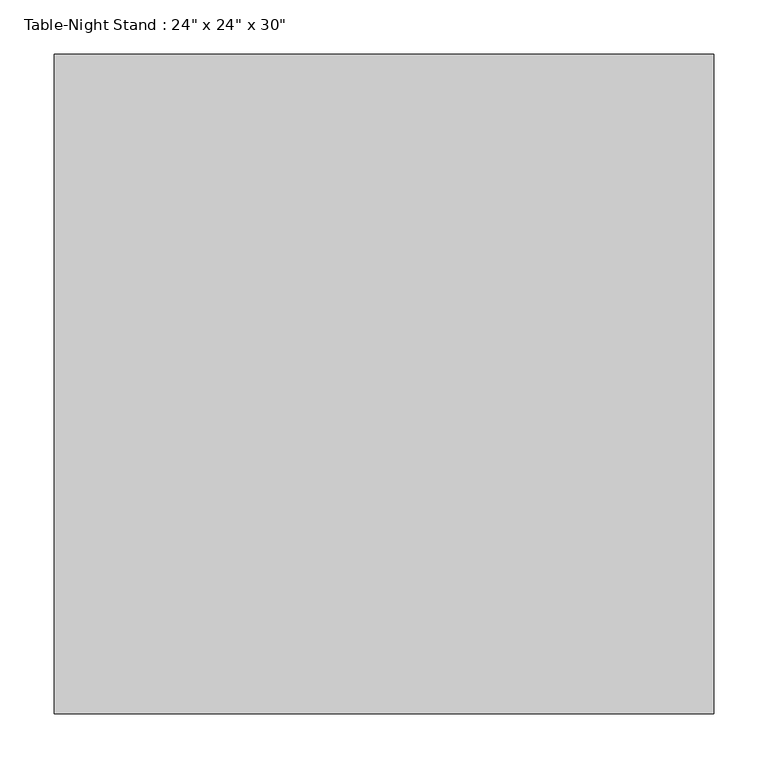
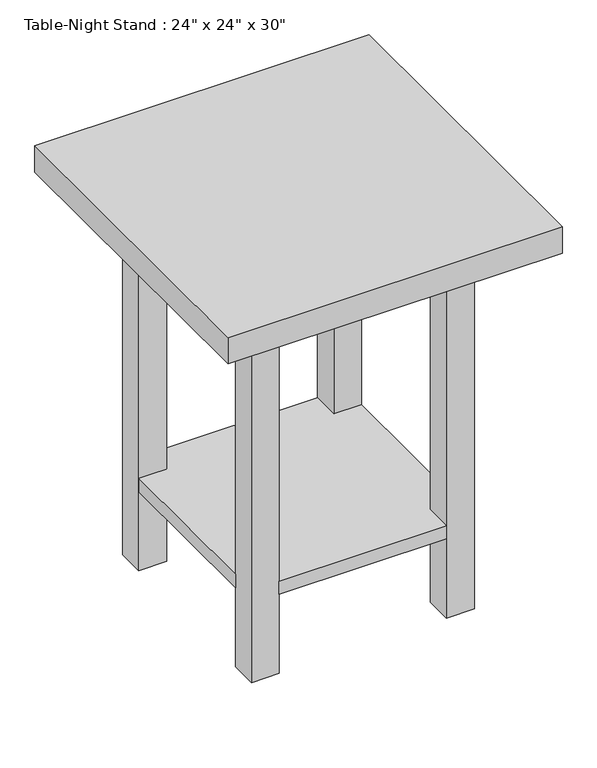
"""IFC4 building model written with IfcOpenShell, lengths in millimetres: furniture geometry."""

from ifc_helpers import new_model, si_unit, frame, origin, origin_with_axes, place, context, project, spatial, polyline, outline, extrude, source, transform, mapped, element, save


def furniture_5bc9ed15(model_context):
    return source(origin(), model_context, "Body", "SweptSolid", [
        extrude(outline(polyline([(156.1336303, 508.0), (460.9336303, 508.0), (460.9336303, 457.2), (511.7336303, 457.2), (511.7336303, 152.4), (460.9336303, 152.4), (460.9336303, 101.6), (156.1336303, 101.6), (156.1336303, 152.4), (105.3336303, 152.4), (105.3336303, 457.2), (156.1336303, 457.2), (156.1336303, 508.0)])), frame((0.0, 0.0, 152.4), z_axis=(0.0, 0.0, 1.0), x_axis=(1.0, 0.0, 0.0)), (0.0, 0.0, 1.0), 25.4),
        extrude(outline(polyline([(156.1336303, 508.0), (156.1336303, 457.2), (105.3336303, 457.2), (105.3336303, 508.0), (156.1336303, 508.0)])), origin_with_axes(), (0.0, 0.0, 1.0), 711.2),
        extrude(outline(polyline([(156.1336303, 152.4), (156.1336303, 101.6), (105.3336303, 101.6), (105.3336303, 152.4), (156.1336303, 152.4)])), origin_with_axes(), (0.0, 0.0, 1.0), 711.2),
        extrude(outline(polyline([(511.7336303, 508.0), (511.7336303, 457.2), (460.9336303, 457.2), (460.9336303, 508.0), (511.7336303, 508.0)])), origin_with_axes(), (0.0, 0.0, 1.0), 711.2),
        extrude(outline(polyline([(511.7336303, 152.4), (511.7336303, 101.6), (460.9336303, 101.6), (460.9336303, 152.4), (511.7336303, 152.4)])), origin_with_axes(), (0.0, 0.0, 1.0), 711.2),
        extrude(outline(polyline([(613.3336303, 0.0), (3.7336303, 0.0), (3.7336303, 609.6), (613.3336303, 609.6), (613.3336303, 0.0)])), frame((0.0, 0.0, 711.2), z_axis=(0.0, 0.0, 1.0), x_axis=(1.0, 0.0, 0.0)), (0.0, 0.0, 1.0), 50.8),
    ])


if __name__ == "__main__":
    model = new_model("IFC4")
    model_context = context("Model", 3, world=origin())
    ifc_project = project(units=[si_unit("LENGTHUNIT", "METRE", prefix="MILLI")], contexts=[model_context])
    site = spatial("IfcSite", under=ifc_project)
    building = spatial("IfcBuilding", under=site)
    placement = place(None, origin())
    furniture_shape = furniture_5bc9ed15(model_context)
    element("IfcFurniture", 1, ObjectType="Table-Night Stand : 24\" x 24\" x 30\"", at=placement, inside=building, context=model_context, shape_type="MappedRepresentation", body=[
        mapped(furniture_shape, transform((0.0, 0.0, 0.0), x_axis=(1.0, 0.0, 0.0), y_axis=(0.0, 1.0, 0.0), z_axis=(0.0, 0.0, 1.0))),
    ])
    save(model, "model.ifc")

# Revit data of these elements
# Type "Table-Night Stand : 24\" x 24\" x 30\""
#   Assembly Code = "E2020200"
#   Depth = 2' - 0"
#   Height = 2' - 6"
#   Width = 2' - 0"
#   Base Material = Birch
#   Top Material = Laminate, Ivory, Matte
#   Default Elevation = 0
# Element 1 (IfcFurniture, "Table-Night Stand : 24\" x 24\" x 30\"")
#   Materials on its faces: "Birch", "Laminate, Ivory, Matte"
# Materials
#   "Birch": class "Wood", colour RGB 210 159 95, transparency 0, Description = "Betula Alleghaniensis", Cost = 0
#   "Laminate, Ivory, Matte": class "Plastic", colour RGB 247 247 239, transparency 0, Description = "Plastic Laminate - Ivory, Matte", Cost = 0
